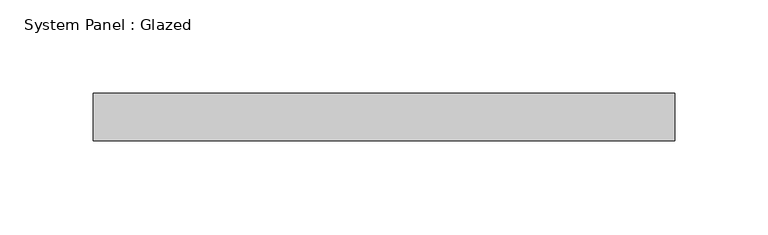
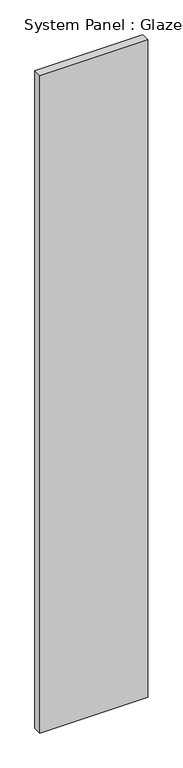
"""IFC4 building model written with IfcOpenShell, lengths in millimetres: plate geometry, System Panel : Glazed."""

from ifc_helpers import new_model, si_unit, origin, origin_with_axes, place, context, project, spatial, polyline, outline, extrude, source, transform, mapped, element, save


def system_panel_glazed_45f6ab2d(model_context):
    return source(origin(), model_context, "Body", "SweptSolid", [
        extrude(outline(polyline([(155.575, 19.05), (-155.575, 19.05), (-155.575, 44.45), (155.575, 44.45), (155.575, 19.05)])), origin_with_axes(), (0.0, 0.0, 1.0), 2006.6),
    ])


if __name__ == "__main__":
    model = new_model("IFC4")
    model_context = context("Model", 3, world=origin())
    ifc_project = project(units=[si_unit("LENGTHUNIT", "METRE", prefix="MILLI")], contexts=[model_context])
    site = spatial("IfcSite", under=ifc_project)
    building = spatial("IfcBuilding", under=site)
    placement = place(None, origin())
    system_panel_glazed_shape = system_panel_glazed_45f6ab2d(model_context)
    element("IfcPlate", 1, ObjectType="System Panel : Glazed", at=placement, inside=building, context=model_context, shape_type="MappedRepresentation", body=[
        mapped(system_panel_glazed_shape, transform((0.0, 0.0, 0.0), x_axis=(1.0, 0.0, 0.0), y_axis=(0.0, 1.0, 0.0), z_axis=(0.0, 0.0, 1.0))),
    ])
    save(model, "model.ifc")

# Revit data of these elements
# Type "System Panel : Glazed"
#   Construction Type Id = "GSP4R"
#   Analytic Construction = "1/8 in Pilkington single glazing"
#   Visual Light Transmittance = 0.9
#   Solar Heat Gain Coefficient = 0.86
#   Heat Transfer Coefficient (U) = 1.18115 BTU/(h·ft²·°F)
#   Define Thermal Properties by = 1
# Element 1 (IfcPlate, "System Panel : Glazed")
#   Materials on its faces: "Glass"
# Materials
#   "Glass": class "Glass", colour RGB 0 128 192, transparency 0.75, Description = "Soda Lime Glass", Cost = 0
